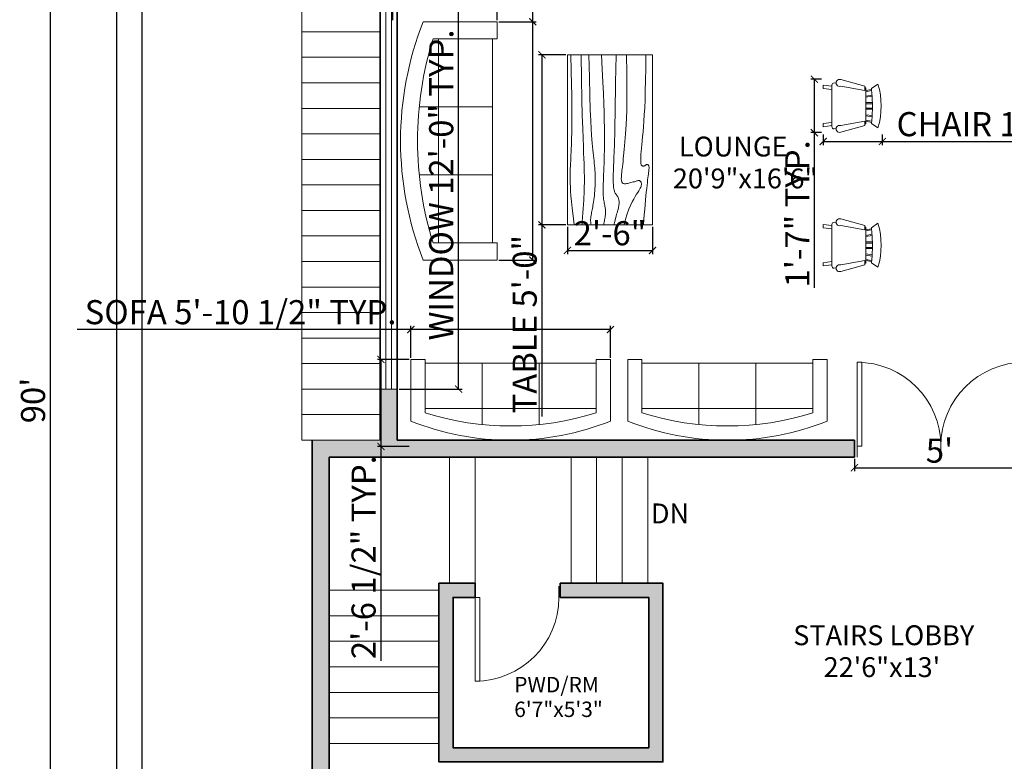
# Model space of a CAD drawing. Units: inches. Extents: x 3799 to 20199, y 1682 to 8087.
# Tile 10 of 30: x 10985 to 11332, y 2537 to 2798. Entities that reach past the tile are written whole.
import ezdxf

# ---------------------------------------------------------------- set-up
doc = ezdxf.new("R2010")
doc.units = ezdxf.units.IN
for name, color, linetype, lineweight in [('A-ANNO-DIMS', 2, 'Continuous', 18), ('A-ANNO-SYMB', 3, 'Continuous', 18), ('A-AREA-IDEN', 7, 'Continuous', 18), ('A-DOOR', 3, 'Continuous', 18), ('A-FLOR-STRS', 41, 'Continuous', 18), ('A-FURN', 8, 'Continuous', 18), ('A-GLAZ', 152, 'Continuous', 18), ('A-WALL', 7, 'Continuous', 35), ('A-WALL-PATT', 252, 'Continuous', 13), ('C-PROP', 7, 'Continuous', 25)]:
    doc.layers.add(name, color=color, linetype=linetype, lineweight=lineweight)
doc.styles.get("Standard").update_dxf_attribs({"font": 'arial.ttf'})
doc.dimstyles.new('ISO-25', dxfattribs={"dimtxt": 8.5, "dimasz": 2.5, "dimexe": 1.25, "dimexo": 0.625, "dimtad": 1, "dimdec": 0, "dimlunit": 3, "dimtxsty": 'Standard', "dimblk": 'ARCHTICK', "dimcen": 2.5, "dimadec": 0, "dimazin": 0, "dimtfac": 1, "dimtdec": 0, "dimtmove": 0, "dimatfit": 3, "dimfxl": 1, "dimarcsym": 0})

# ---------------------------------------------------------------- blocks, each defined once
blk = doc.blocks.new('*U47')
for p, q in [((0, 0), (0, -100)), ((750, 0), (750, -100))]:
    blk.add_line(p, q)
blk.add_lwpolyline([(0, 0), (0, 750), (43.75, 750), (43.75, 0)], close=True)
blk.add_arc((0, 0), 750, 0, 90)
blk = doc.blocks.new('Table - Rectangular Woodgrain 60 x 30 in.')
for p, q in [((0, 0), (0, -30)), ((60, 0), (0, 0)), ((60, -30), (60, 0)), ((0, -30), (60, -30))]:
    blk.add_line(p, q)
for points in [[(0, -2.4), (4.8155, -2.418), (9.0302, -2.4688), (12.709, -2.5477), (15.9167, -2.65), (18.7181, -2.7711), (21.1781, -2.9063), (23.3616, -3.0508), (25.3333, -3.2), (27.1477, -3.3495), (28.8172, -3.4958), (30.3437, -3.636), (31.7291, -3.7667), (32.9756, -3.8849), (34.0849, -3.9875), (35.059, -4.0714), (35.9, -4.1334), (36.6114, -4.1711), (37.2041, -4.1854), (37.6906, -4.1779), (38.0833, -4.15), (38.3948, -4.1034), (38.6375, -4.0396), (38.8239, -3.9602), (38.9666, -3.8667), (39.0764, -3.7608), (39.1573, -3.6448), (39.2116, -3.521), (39.2416, -3.3917), (39.2498, -3.2593), (39.2385, -3.1261), (39.21, -2.9944), (39.1666, -2.8667), (39.111, -2.7447), (39.0468, -2.6281), (38.978, -2.5163), (38.9083, -2.4083), (38.8418, -2.3035), (38.7823, -2.201), (38.7337, -2.1001), (38.7, -2), (38.6844, -1.9003), (38.6875, -1.8021), (38.7094, -1.707), (38.75, -1.6167), (38.8094, -1.5326), (38.8875, -1.4563), (38.9844, -1.3893), (39.1, -1.3333), (39.2351, -1.2896), (39.3937, -1.2583), (39.5804, -1.2396), (39.8, -1.2333), (40.057, -1.2396), (40.3562, -1.2583), (40.7023, -1.2896), (41.1, -1.3333), (41.5547, -1.3895), (42.0755, -1.4573), (42.6721, -1.5361), (43.3542, -1.625), (44.1316, -1.7233), (45.014, -1.8302), (46.0114, -1.9449), (47.1333, -2.0667), (48.3862, -2.1947), (49.7625, -2.3281), (51.2513, -2.4663), (52.8416, -2.6083), (54.5226, -2.7535), (56.2833, -2.9011), (58.1127, -3.0501), (60, -3.2)], [(0, -9.2), (6.5759, -9.0858), (11.9385, -9.0365), (16.2527, -9.0418), (19.6833, -9.0917), (22.3952, -9.1759), (24.5531, -9.2844), (26.322, -9.4069), (27.8666, -9.5333), (29.3241, -9.6553), (30.7203, -9.7719), (32.0532, -9.8837), (33.3208, -9.9917), (34.5213, -10.0965), (35.6526, -10.199), (36.7128, -10.2999), (37.7, -10.4), (38.6129, -10.4996), (39.4531, -10.5969), (40.223, -10.6895), (40.925, -10.775), (41.5613, -10.8512), (42.1344, -10.9156), (42.6465, -10.966), (43.1, -11), (43.4976, -11.0158), (43.8437, -11.0136), (44.143, -10.9942), (44.4, -10.9583), (44.6195, -10.9069), (44.8062, -10.8406), (44.9648, -10.7603), (45.1, -10.6667), (45.2155, -10.5598), (45.3114, -10.4365), (45.3871, -10.2929), (45.4416, -10.125), (45.4743, -9.929), (45.4844, -9.7011), (45.4709, -9.4371), (45.4333, -9.1333), (45.3716, -8.7883), (45.2896, -8.4104), (45.1919, -8.0107), (45.0833, -7.6), (44.9685, -7.1893), (44.8521, -6.7896), (44.7388, -6.4117), (44.6333, -6.0667), (44.54, -5.7628), (44.4614, -5.4979), (44.4001, -5.2675), (44.3583, -5.0667), (44.3384, -4.8909), (44.3427, -4.7354), (44.3736, -4.5956), (44.4333, -4.4667), (44.5236, -4.3453), (44.6427, -4.2333), (44.7884, -4.1339), (44.9583, -4.05), (45.1501, -3.9849), (45.3614, -3.9417), (45.59, -3.9234), (45.8333, -3.9333), (46.0915, -3.9749), (46.3734, -4.0531), (46.6906, -4.1736), (47.0542, -4.3417), (47.4756, -4.5629), (47.9661, -4.8427), (48.5372, -5.1866), (49.2, -5.6), (49.9676, -6.0844), (50.8594, -6.625), (51.8965, -7.2031), (53.1, -7.8), (54.491, -8.3969), (56.0906, -8.975), (57.9199, -9.5156), (60, -10)], [(0, -12.8), (5.1847, -12.9322), (9.6213, -13.0323), (13.3963, -13.1059), (16.5958, -13.1583), (19.3063, -13.1952), (21.614, -13.2219), (23.6054, -13.2439), (25.3666, -13.2667), (26.9728, -13.2947), (28.4531, -13.3281), (29.8256, -13.3663), (31.1083, -13.4083), (32.3191, -13.4535), (33.476, -13.501), (34.597, -13.5501), (35.7, -13.6), (36.7984, -13.6497), (37.8875, -13.6979), (38.9578, -13.743), (40, -13.7833), (41.0047, -13.8174), (41.9625, -13.8438), (42.864, -13.8607), (43.7, -13.8667), (44.4631, -13.8604), (45.1552, -13.8417), (45.7801, -13.8104), (46.3416, -13.7667), (46.8439, -13.7104), (47.2906, -13.6417), (47.6858, -13.5604), (48.0333, -13.4667), (48.3375, -13.3608), (48.6042, -13.2448), (48.8396, -13.121), (49.05, -12.9917), (49.2417, -12.8593), (49.4208, -12.7261), (49.5937, -12.5944), (49.7667, -12.4667), (49.9452, -12.3451), (50.1323, -12.2313), (50.3303, -12.1268), (50.5416, -12.0333), (50.7686, -11.9524), (51.0135, -11.8854), (51.2788, -11.8341), (51.5666, -11.8), (51.8785, -11.7843), (52.2116, -11.7865), (52.562, -11.8059), (52.926, -11.8417), (53.2998, -11.8931), (53.6795, -11.9594), (54.0614, -12.0397), (54.4416, -12.1333), (54.8223, -12.2401), (55.2293, -12.3625), (55.6942, -12.5037), (56.2489, -12.6667), (56.9251, -12.8547), (57.7545, -13.0708), (58.7689, -13.3182), (60, -13.6)], [(0, -18), (5.124, -17.7273), (9.6609, -17.5057), (13.6705, -17.3303), (17.2125, -17.1958), (20.3467, -17.0973), (23.1328, -17.0297), (25.6307, -16.9878), (27.9, -16.9667), (29.9928, -16.9617), (31.9302, -16.9703), (33.7254, -16.9907), (35.3917, -17.0208), (36.9423, -17.0588), (38.3906, -17.1026), (39.7499, -17.1503), (41.0333, -17.2), (42.2519, -17.2496), (43.4073, -17.2969), (44.4986, -17.3395), (45.525, -17.375), (46.4858, -17.4012), (47.3802, -17.4156), (48.2074, -17.416), (48.9667, -17.4), (49.6583, -17.3662), (50.2872, -17.3167), (50.8595, -17.2547), (51.3812, -17.1833), (51.8584, -17.1057), (52.2971, -17.025), (52.7034, -16.9443), (53.0833, -16.8667), (53.443, -16.7951), (53.789, -16.7313), (54.128, -16.6768), (54.4666, -16.6334), (54.8115, -16.6024), (55.1693, -16.5854), (55.5465, -16.5841), (55.95, -16.6), (56.3828, -16.6337), (56.8346, -16.6823), (57.2915, -16.7418), (57.7396, -16.8084), (58.165, -16.878), (58.5539, -16.9469), (58.8924, -17.0111), (59.1666, -17.0667), (59.3679, -17.1107), (59.5078, -17.1438), (59.6032, -17.1675), (59.6708, -17.1833), (59.7275, -17.193), (59.7901, -17.1979), (59.8753, -17.1998), (60, -17.2)], [(0, -22.4), (8.0098, -22.2501), (14.4094, -22.1011), (19.4168, -21.9535), (23.25, -21.8083), (26.1269, -21.6663), (28.2656, -21.5281), (29.884, -21.3947), (31.2, -21.2667), (32.3967, -21.1448), (33.5172, -21.0292), (34.5697, -20.9198), (35.5625, -20.8167), (36.5037, -20.7198), (37.4015, -20.6292), (38.2642, -20.5448), (39.1, -20.4667), (39.9164, -20.3951), (40.7187, -20.3313), (41.5117, -20.2768), (42.3, -20.2333), (43.0883, -20.2024), (43.8812, -20.1854), (44.6836, -20.1841), (45.5, -20.2), (46.3328, -20.234), (47.1747, -20.2844), (48.0163, -20.3488), (48.8479, -20.425), (49.66, -20.5106), (50.4429, -20.6031), (51.1872, -20.7004), (51.8833, -20.8), (52.5246, -20.8999), (53.1166, -20.9995), (53.6681, -21.0983), (54.1875, -21.1958), (54.6834, -21.2919), (55.1646, -21.3859), (55.6394, -21.4777), (56.1167, -21.5667), (56.6028, -21.6515), (57.0961, -21.7266), (57.5929, -21.7852), (58.0896, -21.8208), (58.5823, -21.8268), (59.0674, -21.7964), (59.5412, -21.723), (60, -21.6)], [(0, -25.2), (8.6355, -25.0504), (15.7026, -24.9031), (21.4049, -24.7606), (25.9458, -24.625), (29.529, -24.4988), (32.3578, -24.3844), (34.6359, -24.284), (36.5667, -24.2), (38.3213, -24.1341), (39.9417, -24.0854), (41.437, -24.0523), (42.8167, -24.0333), (44.0901, -24.0268), (45.2667, -24.0313), (46.3557, -24.0451), (47.3667, -24.0667), (48.309, -24.0947), (49.1928, -24.1287), (50.0284, -24.168), (50.826, -24.2125), (51.5959, -24.2617), (52.3483, -24.3151), (53.0935, -24.3725), (53.8417, -24.4334), (54.6009, -24.497), (55.3699, -24.561), (56.1454, -24.6226), (56.9239, -24.6792), (57.7021, -24.7279), (58.4764, -24.7662), (59.2435, -24.7911), (60, -24.8)], [(0, -28.8), (5.6867, -28.6681), (10.45, -28.5698), (14.407, -28.5012), (17.675, -28.4584), (20.3711, -28.4374), (22.6125, -28.4344), (24.5164, -28.4455), (26.2, -28.4667), (27.762, -28.4947), (29.2276, -28.5281), (30.6033, -28.5663), (31.8958, -28.6084), (33.1118, -28.6535), (34.2578, -28.7011), (35.3405, -28.7501), (36.3666, -28.8), (37.3443, -28.8497), (38.288, -28.8974), (39.2137, -28.9412), (40.1375, -28.9792), (41.0753, -29.0093), (42.0432, -29.0297), (43.0572, -29.0384), (44.1333, -29.0333), (45.2936, -29.0114), (46.5843, -28.9641), (48.0579, -28.8816), (49.7666, -28.7542), (51.7629, -28.5721), (54.0989, -28.3255), (56.8272, -28.0048), (60, -27.6)]]:
    blk.add_lwpolyline(points)
blk = doc.blocks.new('Sofa - Roundback 7 ft.')
for p, q in [((-12.00002, -32.4421), (-12.00003, -6.5971)), ((11.99997, -32.4421), (11.99998, -6.5971)), ((-36.000027, -34), (-36.000027, -11.4696)), ((-35.999844, -13.3819), (35.9998, -13.3819)), ((35.99998, -34), (35.99998, -11.4696)), ((-36.000027, -32.4421), (35.99998, -32.4421))]:
    blk.add_line(p, q)
for points in [[(-36.000027, -34), (-42.000027, -34), (-42.000027, -8)], [(41.99998, -8), (41.99998, -34), (35.99998, -34)]]:
    blk.add_lwpolyline(points)
for centre, radius, start, end in [((0, -114.25), 114.25, 68.43141, 111.5686), ((-0.00001, -127.1968), 121.1968, 72.72033, 107.2797)]:
    blk.add_arc(centre, radius, start, end)
blk = doc.blocks.new('_ArchTick')
at = {"color": 0, "linetype": 'ByBlock', "const_width": 0.15}
blk.add_lwpolyline([(-0.5, -0.5), (0.5, 0.5)], dxfattribs=at)
blk = doc.blocks.new('*D77')
at = {"layer": 'A-ANNO-DIMS', "color": 0, "lineweight": -2, "transparency": 16777216}
for p, q in [((11018.23, 3204.07), (10994.27, 3204.07)), ((10995.52, 3204.07), (10995.52, 2124.07)), ((11018.23, 2124.07), (10994.27, 2124.07))]:
    blk.add_line(p, q, dxfattribs=at)
at = {"layer": 'Defpoints', "color": 0, "transparency": 16777216}
for p in [(11018.85, 3204.07), (10995.52, 2124.07), (11018.85, 2124.07)]:
    blk.add_point(p, dxfattribs=at)
at = {"layer": 'A-ANNO-DIMS', "color": 0, "lineweight": -2, "transparency": 16777216, "xscale": 2.5, "yscale": 2.5, "zscale": 2.5}
for p, rotation in [((10995.52, 3204.07), 90), ((10995.52, 2124.07), 270)]:
    blk.add_blockref('_ArchTick', p, dxfattribs=dict(at, rotation=rotation))
at = {"layer": 'A-ANNO-DIMS', "color": 0, "transparency": 16777216, "insert": (10990.56, 2664.07), "char_height": 8.5, "attachment_point": 5, "rotation": 90}
blk.add_mtext("90'", dxfattribs=at)
blk = doc.blocks.new('*U79')
for p, q in [((0, 0), (0, 100)), ((750, 0), (750, 100))]:
    blk.add_line(p, q)
blk.add_lwpolyline([(0, 0), (0, -750), (43.75, -750), (43.75, 0)], close=True)
blk.add_arc((0, 0), 750, 270, 0)
blk = doc.blocks.new('*D80')
at = {"layer": 'A-ANNO-DIMS', "color": 0, "lineweight": -2, "transparency": 16777216}
for p, q in [((11278.96, 2643.45), (11278.96, 2639.11)), ((11338.96, 2643.45), (11338.96, 2639.11)), ((11278.96, 2640.36), (11338.96, 2640.36))]:
    blk.add_line(p, q, dxfattribs=at)
at = {"layer": 'Defpoints', "color": 0, "transparency": 16777216}
for p in [(11278.96, 2644.07), (11338.96, 2644.07), (11338.96, 2640.36)]:
    blk.add_point(p, dxfattribs=at)
at = {"layer": 'A-ANNO-DIMS', "color": 0, "lineweight": -2, "transparency": 16777216, "xscale": 2.5, "yscale": 2.5, "zscale": 2.5, "rotation": 180}
blk.add_blockref('_ArchTick', (11278.96, 2640.36), dxfattribs=at)
at = {"layer": 'A-ANNO-DIMS', "color": 0, "lineweight": -2, "transparency": 16777216, "xscale": 2.5, "yscale": 2.5, "zscale": 2.5}
blk.add_blockref('_ArchTick', (11338.96, 2640.36), dxfattribs=at)
at = {"layer": 'A-ANNO-DIMS', "color": 0, "transparency": 16777216, "insert": (11308.96, 2645.3), "char_height": 8.5, "attachment_point": 5}
blk.add_mtext("5'", dxfattribs=at)
blk = doc.blocks.new('Chair - Rocking')
for p, q in [((-8, -4.5), (-10, -1.5)), ((-6.5, -7), (-7.02225, -4.43)), ((-4.5, -7), (-4.96674, -4.19951)), ((-4, -7), (-4.40532, -4.16272)), ((-1.5, -4.05012), (-1.5, -7)), ((-1, -7), (-1, -4.05012)), ((1, -7), (1, -4.04655)), ((1.5, -4.05012), (1.5, -7)), ((4, -7), (4.40187, -4.18694)), ((4.5, -7), (4.96761, -4.19437)), ((6.5, -7), (7, -4.4057)), ((8, -4.5), (10, -1.5)), ((-9, -7.5), (-12, -18.49999)), ((-7, -7.5), (-9, -7.5)), ((-9, -18.49999), (-7, -7.5)), ((-8.23428, -6.99939), (-8.3093, -7.47958)), ((-8.23041, -7), (8.23915, -7)), ((-7.5, -4.5), (-7, -7)), ((7.5, -4.5), (7, -7)), ((7, -7.5), (9, -7.5)), ((9, -18.49999), (7, -7.5)), ((8.31071, -7.48854), (8.23449, -7.00073)), ((9, -7.5), (12, -18.49999)), ((-10.36644, -20.64523), (-10.5, -21.49999)), ((10.5, -21.49999), (10.3575, -20.58798)), ((-9, -22.49999), (-9.5, -26.49999)), ((0, -22.49999), (-9.5, -22.49999)), ((-9.5, -26.49999), (-8, -26.49999)), ((-8, -26.49999), (-7.5, -22.49999)), ((0, -22.49999), (9.5, -22.49999)), ((8, -26.49999), (7.5, -22.49999)), ((9.5, -26.49999), (8, -26.49999)), ((9, -22.49999), (9.5, -26.49999))]:
    blk.add_line(p, q)
for centre, radius, start, end in [((0, -34.08333), 34.08333, 72.93847, 107.0615), ((0, -68.25004), 64.25, 93.92211, 97.15267), ((0, -68.25004), 64.25, 82.84733, 93.92211), ((-10.5, -18.99999), 1.58114, 161.5651, 18.43495), ((-9.5, -21.49999), 1, 180, 270), ((10.5, -18.99999), 1.58114, 161.5651, 18.43495), ((9.5, -21.49999), 1, 270, 0)]:
    blk.add_arc(centre, radius, start, end)
blk = doc.blocks.new('WIN-144IN-6IN-FRAME')
for p, q in [((0, 6), (0, 0)), ((144, 4), (0, 4)), ((144, 6), (144, 0)), ((144, 2), (0, 2))]:
    blk.add_line(p, q)
blk = doc.blocks.new('*D258')
at = {"layer": 'A-ANNO-DIMS', "color": 0, "lineweight": -2, "transparency": 16777216}
for p, q in [((11165.6, 2797.6), (11165.6, 2888.75)), ((11153.62, 2797.6), (11166.85, 2797.6)), ((11165.6, 2713.6), (11165.6, 2797.6)), ((11153.62, 2713.6), (11166.85, 2713.6))]:
    blk.add_line(p, q, dxfattribs=at)
at = {"layer": 'Defpoints', "color": 0, "transparency": 16777216}
for p in [(11153, 2797.6), (11165.6, 2797.6), (11153, 2713.6)]:
    blk.add_point(p, dxfattribs=at)
at = {"layer": 'A-ANNO-DIMS', "color": 0, "lineweight": -2, "transparency": 16777216, "xscale": 2.5, "yscale": 2.5, "zscale": 2.5}
for p, rotation in [((11165.6, 2797.6), 90), ((11165.6, 2713.6), 270)]:
    blk.add_blockref('_ArchTick', p, dxfattribs=dict(at, rotation=rotation))
at = {"layer": 'A-ANNO-DIMS', "color": 0, "transparency": 16777216, "insert": (11160.58, 2844.42), "char_height": 8.5, "attachment_point": 5, "rotation": 90}
blk.add_mtext('SOFA 7\'-0" TYP.', dxfattribs=at)
blk = doc.blocks.new('*D259')
at = {"layer": 'A-ANNO-DIMS', "color": 0, "lineweight": -2, "transparency": 16777216}
for p, q in [((11116.33, 2798.22), (11116.33, 2811.45)), ((11153, 2798.22), (11153, 2811.45)), ((11116.33, 2810.2), (11040.97, 2810.2)), ((11153, 2810.2), (11116.33, 2810.2))]:
    blk.add_line(p, q, dxfattribs=at)
at = {"layer": 'Defpoints', "color": 0, "transparency": 16777216}
for p in [(11116.33, 2810.2), (11116.33, 2797.6), (11153, 2797.6)]:
    blk.add_point(p, dxfattribs=at)
at = {"layer": 'A-ANNO-DIMS', "color": 0, "lineweight": -2, "transparency": 16777216, "xscale": 2.5, "yscale": 2.5, "zscale": 2.5, "rotation": 180}
blk.add_blockref('_ArchTick', (11116.33, 2810.2), dxfattribs=at)
at = {"layer": 'A-ANNO-DIMS', "color": 0, "lineweight": -2, "transparency": 16777216, "xscale": 2.5, "yscale": 2.5, "zscale": 2.5}
blk.add_blockref('_ArchTick', (11153, 2810.2), dxfattribs=at)
at = {"layer": 'A-ANNO-DIMS', "color": 0, "transparency": 16777216, "insert": (11077.4, 2815.22), "char_height": 8.5, "attachment_point": 5}
blk.add_mtext('3\'-0 1/2" TYP.', dxfattribs=at)
blk = doc.blocks.new('*D260')
at = {"layer": 'A-ANNO-DIMS', "color": 0, "lineweight": -2, "transparency": 16777216}
for p, q in [((11122.64, 2679.16), (11122.64, 2690.34)), ((11192.97, 2679.16), (11192.97, 2690.34)), ((11122.64, 2689.09), (11005.08, 2689.09)), ((11192.97, 2689.09), (11122.64, 2689.09))]:
    blk.add_line(p, q, dxfattribs=at)
at = {"layer": 'Defpoints', "color": 0, "transparency": 16777216}
for p in [(11122.64, 2689.09), (11122.64, 2678.54), (11192.97, 2678.54)]:
    blk.add_point(p, dxfattribs=at)
at = {"layer": 'A-ANNO-DIMS', "color": 0, "lineweight": -2, "transparency": 16777216, "xscale": 2.5, "yscale": 2.5, "zscale": 2.5, "rotation": 180}
blk.add_blockref('_ArchTick', (11122.64, 2689.09), dxfattribs=at)
at = {"layer": 'A-ANNO-DIMS', "color": 0, "lineweight": -2, "transparency": 16777216, "xscale": 2.5, "yscale": 2.5, "zscale": 2.5}
blk.add_blockref('_ArchTick', (11192.97, 2689.09), dxfattribs=at)
at = {"layer": 'A-ANNO-DIMS', "color": 0, "transparency": 16777216, "insert": (11062.61, 2694.11), "char_height": 8.5, "attachment_point": 5}
blk.add_mtext('SOFA 5\'-10 1/2" TYP.', dxfattribs=at)
blk = doc.blocks.new('*D261')
at = {"layer": 'A-ANNO-DIMS', "color": 0, "lineweight": -2, "transparency": 16777216}
for p, q in [((11122.01, 2678.54), (11110.84, 2678.54)), ((11112.09, 2678.54), (11112.09, 2647.84)), ((11122.01, 2647.84), (11110.84, 2647.84)), ((11112.09, 2647.84), (11112.09, 2572.33))]:
    blk.add_line(p, q, dxfattribs=at)
at = {"layer": 'Defpoints', "color": 0, "transparency": 16777216}
for p in [(11122.64, 2678.54), (11112.09, 2647.84), (11122.64, 2647.84)]:
    blk.add_point(p, dxfattribs=at)
at = {"layer": 'A-ANNO-DIMS', "color": 0, "lineweight": -2, "transparency": 16777216, "xscale": 2.5, "yscale": 2.5, "zscale": 2.5}
for p, rotation in [((11112.09, 2678.54), 90), ((11112.09, 2647.84), 270)]:
    blk.add_blockref('_ArchTick', p, dxfattribs=dict(at, rotation=rotation))
at = {"layer": 'A-ANNO-DIMS', "color": 0, "transparency": 16777216, "insert": (11107.07, 2608.83), "char_height": 8.5, "attachment_point": 5, "rotation": 90}
blk.add_mtext('2\'-6 1/2" TYP.', dxfattribs=at)
blk = doc.blocks.new('*D316')
at = {"layer": 'A-ANNO-DIMS', "color": 0, "lineweight": -2, "transparency": 16777216}
for p, q in [((11267.96, 2757.88), (11267.96, 2754.13)), ((11288.8, 2757.88), (11288.8, 2754.13)), ((11267.96, 2755.38), (11288.8, 2755.38)), ((11288.8, 2755.38), (11384.5, 2755.38))]:
    blk.add_line(p, q, dxfattribs=at)
at = {"layer": 'Defpoints', "color": 0, "transparency": 16777216}
for p in [(11267.96, 2758.5), (11288.8, 2758.5), (11288.8, 2755.38)]:
    blk.add_point(p, dxfattribs=at)
at = {"layer": 'A-ANNO-DIMS', "color": 0, "lineweight": -2, "transparency": 16777216, "xscale": 2.5, "yscale": 2.5, "zscale": 2.5, "rotation": 180}
blk.add_blockref('_ArchTick', (11267.96, 2755.38), dxfattribs=at)
at = {"layer": 'A-ANNO-DIMS', "color": 0, "lineweight": -2, "transparency": 16777216, "xscale": 2.5, "yscale": 2.5, "zscale": 2.5}
blk.add_blockref('_ArchTick', (11288.8, 2755.38), dxfattribs=at)
at = {"layer": 'A-ANNO-DIMS', "color": 0, "transparency": 16777216, "insert": (11337.9, 2760.4), "char_height": 8.5, "attachment_point": 5}
blk.add_mtext('CHAIR 1\'-9" TYP.', dxfattribs=at)
blk = doc.blocks.new('*D317')
at = {"layer": 'A-ANNO-DIMS', "color": 0, "lineweight": -2, "transparency": 16777216}
for p, q in [((11267.33, 2777.36), (11263.58, 2777.36)), ((11264.83, 2777.36), (11264.83, 2758.5)), ((11267.33, 2758.5), (11263.58, 2758.5)), ((11264.83, 2758.5), (11264.83, 2703.74))]:
    blk.add_line(p, q, dxfattribs=at)
at = {"layer": 'Defpoints', "color": 0, "transparency": 16777216}
for p in [(11267.96, 2777.36), (11264.83, 2758.5), (11267.96, 2758.5)]:
    blk.add_point(p, dxfattribs=at)
at = {"layer": 'A-ANNO-DIMS', "color": 0, "lineweight": -2, "transparency": 16777216, "xscale": 2.5, "yscale": 2.5, "zscale": 2.5}
for p, rotation in [((11264.83, 2777.36), 90), ((11264.83, 2758.5), 270)]:
    blk.add_blockref('_ArchTick', p, dxfattribs=dict(at, rotation=rotation))
at = {"layer": 'A-ANNO-DIMS', "color": 0, "transparency": 16777216, "insert": (11259.94, 2729.87), "char_height": 8.5, "attachment_point": 5, "rotation": 90}
blk.add_mtext('1\'-7" TYP.', dxfattribs=at)
blk = doc.blocks.new('*D330')
at = {"layer": 'A-ANNO-DIMS', "color": 0, "lineweight": -2, "transparency": 16777216}
for p, q in [((11177.2, 2785.96), (11167.57, 2785.96)), ((11168.82, 2785.96), (11168.82, 2725.96)), ((11177.2, 2725.96), (11167.57, 2725.96)), ((11168.82, 2725.96), (11168.82, 2658.48))]:
    blk.add_line(p, q, dxfattribs=at)
at = {"layer": 'Defpoints', "color": 0, "transparency": 16777216}
for p in [(11177.82, 2785.96), (11168.82, 2725.96), (11177.82, 2725.96)]:
    blk.add_point(p, dxfattribs=at)
at = {"layer": 'A-ANNO-DIMS', "color": 0, "lineweight": -2, "transparency": 16777216, "xscale": 2.5, "yscale": 2.5, "zscale": 2.5}
for p, rotation in [((11168.82, 2785.96), 90), ((11168.82, 2725.96), 270)]:
    blk.add_blockref('_ArchTick', p, dxfattribs=dict(at, rotation=rotation))
at = {"layer": 'A-ANNO-DIMS', "color": 0, "transparency": 16777216, "insert": (11163.86, 2690.97), "char_height": 8.5, "attachment_point": 5, "rotation": 90}
blk.add_mtext('TABLE 5\'-0"', dxfattribs=at)
blk = doc.blocks.new('*D331')
at = {"layer": 'A-ANNO-DIMS', "color": 0, "lineweight": -2, "transparency": 16777216}
for p, q in [((11177.82, 2725.34), (11177.82, 2715.71)), ((11207.82, 2725.34), (11207.82, 2715.71)), ((11177.82, 2716.96), (11207.82, 2716.96))]:
    blk.add_line(p, q, dxfattribs=at)
at = {"layer": 'Defpoints', "color": 0, "transparency": 16777216}
for p in [(11177.82, 2725.96), (11207.82, 2725.96), (11207.82, 2716.96)]:
    blk.add_point(p, dxfattribs=at)
at = {"layer": 'A-ANNO-DIMS', "color": 0, "lineweight": -2, "transparency": 16777216, "xscale": 2.5, "yscale": 2.5, "zscale": 2.5, "rotation": 180}
blk.add_blockref('_ArchTick', (11177.82, 2716.96), dxfattribs=at)
at = {"layer": 'A-ANNO-DIMS', "color": 0, "lineweight": -2, "transparency": 16777216, "xscale": 2.5, "yscale": 2.5, "zscale": 2.5}
blk.add_blockref('_ArchTick', (11207.82, 2716.96), dxfattribs=at)
at = {"layer": 'A-ANNO-DIMS', "color": 0, "transparency": 16777216, "insert": (11192.82, 2721.93), "char_height": 8.5, "attachment_point": 5}
blk.add_mtext('2\'-6"', dxfattribs=at)
blk = doc.blocks.new('*D354')
at = {"layer": 'A-ANNO-DIMS', "color": 0, "lineweight": -2, "transparency": 16777216}
for p, q in [((11118.48, 2812.07), (11140.7, 2812.07)), ((11139.45, 2668.07), (11139.45, 2812.07)), ((11118.48, 2668.07), (11140.7, 2668.07))]:
    blk.add_line(p, q, dxfattribs=at)
at = {"layer": 'Defpoints', "color": 0, "transparency": 16777216}
for p in [(11117.85, 2812.07), (11139.45, 2812.07), (11117.85, 2668.07)]:
    blk.add_point(p, dxfattribs=at)
at = {"layer": 'A-ANNO-DIMS', "color": 0, "lineweight": -2, "transparency": 16777216, "xscale": 2.5, "yscale": 2.5, "zscale": 2.5}
for p, rotation in [((11139.45, 2812.07), 90), ((11139.45, 2668.07), 270)]:
    blk.add_blockref('_ArchTick', p, dxfattribs=dict(at, rotation=rotation))
at = {"layer": 'A-ANNO-DIMS', "color": 0, "transparency": 16777216, "insert": (11134.43, 2740.07), "char_height": 8.5, "attachment_point": 5, "rotation": 90}
blk.add_mtext('WINDOW 12\'-0" TYP.', dxfattribs=at)

msp = doc.modelspace()

# ---------------------------------------------------------------- hatches: boundary and pattern name
at = {"layer": 'A-WALL-PATT'}
h = msp.add_hatch(color=256, dxfattribs=at)
h.dxf.hatch_style = 1
h.paths.add_polyline_path([(11549.85, 2537.07), (11543.85, 2537.07), (11543.85, 2493.07), (11500.92, 2493.07), (11500.92, 2487.07), (11543.85, 2487.07), (11543.85, 2331.07), (11512.59, 2331.07), (11512.59, 2325.07), (11549.85, 2325.07)])
h.paths.add_polyline_path([(11404.92, 2493.07), (11369.85, 2493.07), (11369.85, 2535.29), (11363.85, 2535.29), (11363.85, 2493.07), (11359.67, 2493.07), (11359.67, 2487.07), (11404.92, 2487.07)])
h.paths.add_polyline_path([(11347.67, 2493.07), (11315.85, 2493.07), (11315.85, 2481.32), (11321.85, 2481.32), (11321.85, 2487.07), (11347.67, 2487.07)])
h.paths.add_polyline_path([(11246.96, 2394.07), (11231.85, 2394.07), (11231.85, 2493.07), (11126.81, 2493.07), (11126.81, 2487.07), (11225.85, 2487.07), (11225.85, 2325.07), (11315.85, 2325.07), (11315.85, 2331.07), (11231.85, 2331.07), (11231.85, 2388.07), (11246.96, 2388.07)])
h.paths.add_polyline_path([(11368.59, 2331.07), (11321.85, 2331.07), (11321.85, 2421.32), (11319.79, 2421.32), (11315.85, 2421.32), (11315.85, 2394.07), (11306.96, 2394.07), (11306.96, 2392.01), (11306.96, 2388.07), (11315.85, 2388.07), (11315.85, 2325.07), (11368.59, 2325.07)])
h.paths.add_polyline_path([(11211.5, 2599.62), (11175.25, 2599.62), (11175.25, 2594.62), (11206.5, 2594.62), (11206.5, 2541.62), (11137.5, 2541.62), (11137.5, 2594.62), (11145.25, 2594.62), (11145.25, 2599.62), (11132.5, 2599.62), (11132.5, 2536.62), (11211.5, 2536.62)], flags=17)
h.paths.add_polyline_path([(11278.96, 2650.07), (11117.85, 2650.07), (11117.85, 2668.07), (11111.85, 2668.07), (11111.85, 2650.07), (11087.85, 2650.07), (11087.85, 2526.57), (11093.85, 2526.57), (11093.85, 2644.07), (11278.96, 2644.07)])
h.paths.add_polyline_path([(11096.81, 2491.01), (11096.81, 2493.07), (11093.85, 2493.07), (11093.85, 2496.57), (11087.85, 2496.57), (11087.85, 2487.07), (11096.81, 2487.07)])
h.paths.add_polyline_path([(11445.85, 3087.71), (11439.85, 3087.71), (11439.85, 2949.07), (11343.85, 2949.07), (11343.85, 2929.61), (11315.6, 2929.61), (11315.6, 2923.61), (11343.85, 2923.61), (11343.85, 2840.12), (11349.85, 2840.12), (11349.85, 2943.07), (11507.11, 2943.07), (11507.11, 2949.07), (11445.85, 2949.07), (11445.85, 3015.07), (11543.85, 3015.07), (11543.85, 2992.92), (11549.85, 2992.92), (11549.85, 3108.28), (11543.85, 3108.28), (11543.85, 3021.07), (11515.89, 3021.07), (11515.89, 3049.36), (11511.89, 3049.36), (11511.89, 3021.07), (11445.85, 3021.07)])
h.paths.add_polyline_path([(11549.85, 3135.07), (11408.12, 3135.07), (11408.12, 3129.07), (11439.85, 3129.07), (11439.85, 3117.71), (11443.79, 3117.71), (11445.85, 3117.71), (11445.85, 3129.07), (11504.47, 3129.07), (11504.47, 3099.65), (11508.47, 3099.65), (11508.47, 3129.07), (11543.85, 3129.07), (11543.85, 3126.28), (11549.85, 3126.28)])
h.paths.add_polyline_path([(11324.12, 3135.07), (11087.85, 3135.07), (11087.85, 3083.46), (11093.85, 3083.46), (11093.85, 3129.07), (11265.85, 3129.07), (11265.85, 3050.07), (11240.75, 3050.07), (11240.75, 3044.07), (11265.85, 3044.07), (11265.85, 2895.64), (11271.85, 2895.64), (11271.85, 2923.61), (11279.6, 2923.61), (11279.6, 2929.61), (11271.85, 2929.61), (11271.85, 3129.07), (11324.12, 3129.07)])
h.paths.add_polyline_path([(11210.75, 3050.07), (11133.85, 3050.07), (11133.85, 3088.63), (11129.85, 3088.54), (11129.85, 3050.07), (11093.85, 3050.07), (11093.85, 3059.46), (11087.85, 3059.46), (11087.85, 3030.25), (11093.85, 3030.25), (11093.85, 3044.07), (11210.75, 3044.07)], flags=17)
h.paths.add_polyline_path([(11093.85, 2982.25), (11087.85, 2982.25), (11087.85, 2913.95), (11093.85, 2913.95)], flags=17)
h.paths.add_polyline_path([(11271.85, 2859.64), (11265.85, 2859.64), (11265.85, 2854.07), (11093.85, 2854.07), (11093.85, 2865.95), (11087.85, 2865.95), (11087.85, 2848.07), (11111.85, 2848.07), (11111.85, 2812.07), (11117.85, 2812.07), (11117.85, 2848.07), (11271.85, 2848.07)])
h.paths.add_polyline_path([(11549.85, 2847.23), (11543.85, 2847.23), (11543.85, 2799.07), (11349.85, 2799.07), (11349.85, 2804.12), (11343.85, 2804.12), (11343.85, 2753.07), (11349.85, 2753.07), (11349.85, 2793.07), (11543.85, 2793.07), (11543.85, 2752.31), (11549.85, 2752.31)])
h.paths.add_polyline_path([(11549.85, 2692.31), (11543.85, 2692.31), (11543.85, 2650.07), (11343.85, 2650.07), (11338.96, 2650.07), (11338.96, 2644.07), (11349.85, 2644.07), (11363.85, 2644.07), (11363.85, 2608.29), (11369.85, 2608.29), (11369.85, 2644.07), (11543.85, 2644.07), (11543.85, 2621.07), (11549.85, 2621.07)])

# ---------------------------------------------------------------- linework, layer by layer
at = {"layer": 'A-FLOR-STRS'}
for p, q in [((11084.17, 2650.07), (11084.17, 2830.07)), ((11111.85, 2794.07), (11084.17, 2794.07)), ((11111.85, 2785.07), (11084.17, 2785.07)), ((11111.85, 2776.07), (11084.17, 2776.07)), ((11111.85, 2767.07), (11084.17, 2767.07)), ((11111.85, 2758.07), (11084.17, 2758.07)), ((11111.85, 2749.07), (11084.17, 2749.07)), ((11111.85, 2740.07), (11084.17, 2740.07)), ((11111.85, 2731.07), (11084.17, 2731.07)), ((11111.85, 2722.07), (11084.17, 2722.07)), ((11111.85, 2713.07), (11084.17, 2713.07)), ((11111.85, 2704.07), (11084.17, 2704.07)), ((11111.85, 2695.07), (11084.17, 2695.07)), ((11111.85, 2686.07), (11084.17, 2686.07)), ((11111.85, 2677.07), (11084.17, 2677.07)), ((11111.85, 2668.07), (11084.17, 2668.07)), ((11111.85, 2659.07), (11084.17, 2659.07)), ((11111.85, 2650.07), (11084.17, 2650.07)), ((11136.25, 2599.62), (11136.25, 2644.07)), ((11145.25, 2599.62), (11145.25, 2644.07)), ((11179.12, 2599.62), (11179.12, 2644.07)), ((11188.12, 2599.62), (11188.12, 2644.07)), ((11197.12, 2599.62), (11197.12, 2644.07)), ((11206.12, 2599.62), (11206.12, 2644.07)), ((11132.5, 2597.16), (11093.85, 2597.16)), ((11132.5, 2588.16), (11093.85, 2588.16)), ((11132.5, 2579.16), (11093.85, 2579.16)), ((11132.5, 2570.16), (11093.85, 2570.16)), ((11132.5, 2561.16), (11093.85, 2561.16)), ((11132.5, 2552.16), (11093.85, 2552.16)), ((11132.5, 2543.16), (11093.85, 2543.16))]:
    msp.add_line(p, q, dxfattribs=at)
at = {"layer": 'A-WALL'}
for p, q in [((11111.85, 2848.07), (11111.85, 2650.07)), ((11117.85, 2848.07), (11117.85, 2650.07)), ((11087.85, 2650.07), (11087.85, 2487.07)), ((11278.96, 2650.07), (11117.85, 2650.07)), ((11278.96, 2650.07), (11278.96, 2644.07)), ((11093.85, 2644.07), (11093.85, 2493.07)), ((11278.96, 2644.07), (11093.85, 2644.07)), ((11145.25, 2599.62), (11145.25, 2594.62)), ((11175.25, 2599.62), (11175.25, 2594.62))]:
    msp.add_line(p, q, dxfattribs=at)
for points in [[(11175.25, 2599.62), (11211.5, 2599.62), (11211.5, 2536.62), (11132.5, 2536.62), (11132.5, 2599.62), (11145.25, 2599.62)], [(11175.25, 2594.62), (11206.5, 2594.62), (11206.5, 2541.62), (11137.5, 2541.62), (11137.5, 2594.62), (11145.25, 2594.62)]]:
    msp.add_lwpolyline(points, dxfattribs=at)
at = {"layer": 'C-PROP'}
for p, q in [((11018.85, 3204.07), (11018.85, 2124.07)), ((11027.85, 3195.07), (11027.85, 2133.07))]:
    msp.add_line(p, q, dxfattribs=at)

# ---------------------------------------------------------------- block references
at = {"layer": 'A-DOOR', "yscale": 0.0393700787401575, "zscale": 0.0393700787401575}
for name, p, xscale in [('*U47', (11279.91, 2648.01), 0.0393700787401575), ('*U47', (11338.96, 2648.01), -0.0393700787401575), ('*U79', (11145.25, 2594.62), 0.0393700787401575)]:
    msp.add_blockref(name, p, dxfattribs=dict(at, xscale=xscale))
at = {"layer": 'A-FURN'}
for name, p, rotation in [('Sofa - Roundback 7 ft.', (11119, 2755.6), 89.99999999999999), ('Table - Rectangular Woodgrain 60 x 30 in.', (11207.82, 2785.96), 270)]:
    msp.add_blockref(name, p, dxfattribs=dict(at, rotation=rotation))
for name, p, xscale, yscale, zscale, rotation in [('Chair - Rocking', (11288.41, 2767.93), 0.7717321187378473, 0.7717321187378473, 0.7717321187378473, 270.0000000000017), ('Chair - Rocking', (11288.41, 2718.82), 0.7717321187378473, 0.7717321187378473, 0.7717321187378473, 270.0000000000017), ('Sofa - Roundback 7 ft.', (11157.8, 2650.07), 0.8372446880612686, 0.8372446880612686, 0.8372446880612686, 180), ('Sofa - Roundback 7 ft.', (11234.22, 2650.07), 0.8372446880612686, 0.8372446880612686, 0.8372446880612686, 180)]:
    msp.add_blockref(name, p, dxfattribs=dict(at, xscale=xscale, yscale=yscale, zscale=zscale, rotation=rotation))
at = {"layer": 'A-GLAZ', "rotation": 90}
msp.add_blockref('WIN-144IN-6IN-FRAME', (11117.85, 2668.07), dxfattribs=at)

# ---------------------------------------------------------------- texts
at = {"layer": 'A-ANNO-SYMB'}
msp.add_text('DN', height=7, rotation=0.0019, dxfattribs=at).set_placement((11207.24, 2620.75))
at = {"layer": 'A-AREA-IDEN'}
for s, height, p in [(' LOUNGE', 7, (11214.98, 2750.1)), ('20\'9"x16\'6"', 7, (11214.98, 2738.86)), ('STAIRS LOBBY', 7, (11257.41, 2577.79)), ('     22\'6"x13\'', 7, (11257.42, 2566.55)), ('PWD/RM', 5.421, (11159.06, 2561.18)), ('6\'7"x5\'3"', 5.421, (11159.06, 2552.47))]:
    msp.add_text(s, height=height, rotation=0.0019, dxfattribs=at).set_placement(p)

# ---------------------------------------------------------------- dimensions: what is measured, and where the dimension line sits
at = {"layer": 'A-ANNO-DIMS'}
dim = msp.add_linear_dim(base=(10995.52, 2124.07), p1=(11018.85, 3204.07), p2=(11018.85, 2124.07), angle=90, dimstyle='ISO-25', override={"dimclrd": 0, "dimclre": 0, "dimclrt": 0}, dxfattribs=at)
dim.commit()
dim.dimension.update_dxf_attribs({"geometry": '*D77', "text_midpoint": (10990.56, 2664.07)})
for base, p1, p2, angle, text, picture, middle in [((11165.6, 2797.6), (11153, 2713.6), (11153, 2797.6), 90, 'SOFA <> TYP.', '*D258', (11160.58, 2844.42)), ((11116.33, 2810.2), (11153, 2797.6), (11116.33, 2797.6), 180, '<> TYP.', '*D259', (11077.4, 2815.22)), ((11139.45, 2812.07), (11117.85, 2668.07), (11117.85, 2812.07), 90, 'WINDOW <> TYP.', '*D354', (11134.43, 2740.07)), ((11168.82, 2725.96), (11177.82, 2785.96), (11177.82, 2725.96), 270, 'TABLE <>', '*D330', (11163.86, 2690.97)), ((11288.8, 2755.38), (11267.96, 2758.5), (11288.8, 2758.5), 0, 'CHAIR <> TYP.', '*D316', (11337.9, 2760.4)), ((11264.83, 2758.5), (11267.96, 2777.36), (11267.96, 2758.5), 270, '<> TYP.', '*D317', (11259.94, 2729.87)), ((11122.64, 2689.09), (11192.97, 2678.54), (11122.64, 2678.54), 180, 'SOFA <> TYP.', '*D260', (11062.61, 2694.11)), ((11112.09, 2647.84), (11122.64, 2678.54), (11122.64, 2647.84), 270, '<> TYP.', '*D261', (11107.07, 2608.83))]:
    dim = msp.add_linear_dim(base=base, p1=p1, p2=p2, angle=angle, text=text, dimstyle='ISO-25', override={"dimdec": 1, "dimlfac": 1, "dimrnd": 0, "dimzin": 1, "dimdsep": 46, "dimlunit": 4, "dimfrac": 2}, dxfattribs=at)
    dim.commit()
    dim.dimension.update_dxf_attribs({"geometry": picture, "text_midpoint": middle})
for base, p1, p2, override, picture, middle in [((11207.82, 2716.96), (11177.82, 2725.96), (11207.82, 2725.96), {"dimdec": 1, "dimlfac": 1, "dimrnd": 0, "dimzin": 1, "dimdsep": 46, "dimlunit": 4, "dimfrac": 2}, '*D331', (11192.82, 2721.93)), ((11338.96, 2640.36), (11278.96, 2644.07), (11338.96, 2644.07), {"dimclrd": 0, "dimclre": 0, "dimclrt": 0}, '*D80', (11308.96, 2645.3))]:
    dim = msp.add_linear_dim(base=base, p1=p1, p2=p2, dimstyle='ISO-25', override=override, dxfattribs=at)
    dim.commit()
    dim.dimension.update_dxf_attribs({"geometry": picture, "text_midpoint": middle})

doc.saveas('drawing.dxf')
